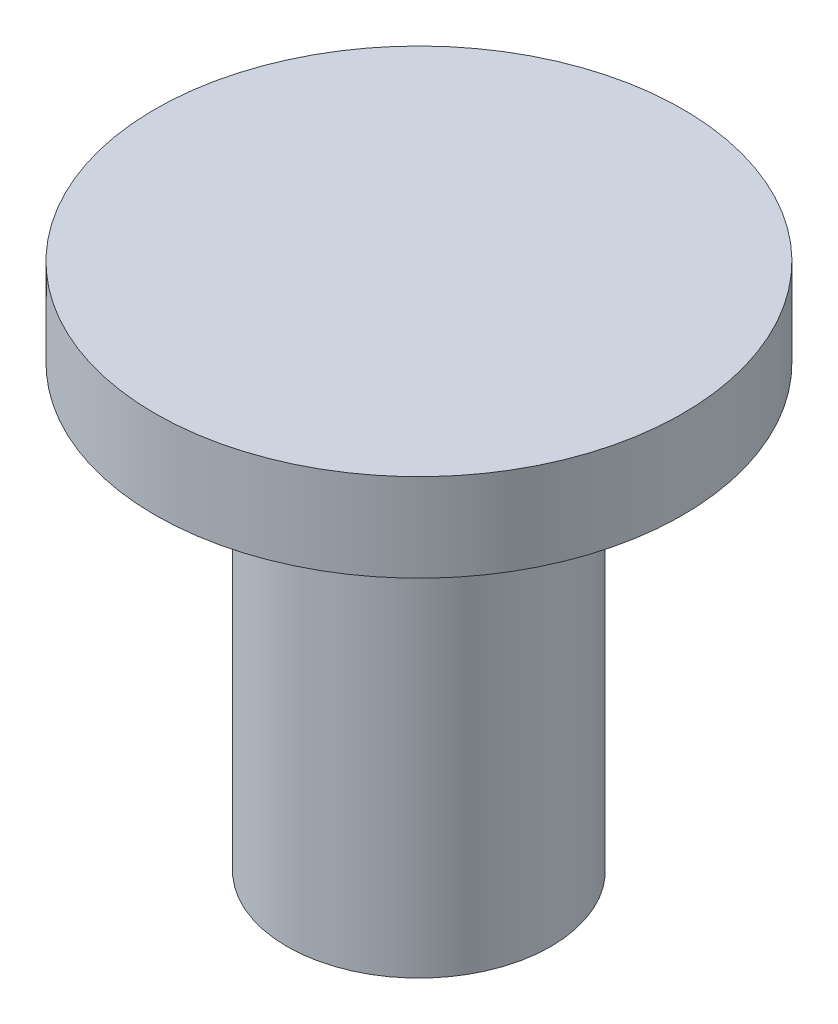
from build123d import *

# Parameters (mm, degrees)
SHANK_PROFILE_6_R = 3
SHANK_6X10_DEPTH  = 10
HEAD_PROFILE_12_R = 6
HEAD_12X2_DEPTH   = 2


with BuildPart() as part:
    # Shank Profile Ø6 → Shank Ø6x10 (new body)
    with BuildSketch(Plane(origin=(0, 0, 0), x_dir=(1, 0, 0), z_dir=(0, 1, 0))):
        with Locations(Location((0, 0, 0), (0, 0, 270))):
            Circle(SHANK_PROFILE_6_R)
    extrude(amount=SHANK_6X10_DEPTH)

    # Head Profile Ø12 → Head Ø12x2 (add)
    with BuildSketch(Plane(origin=(0, 10, 0), x_dir=(1, 0, 0), z_dir=(0, 1, 0))):
        with Locations(Location((0, 0, 0), (0, 0, 270))):
            Circle(HEAD_PROFILE_12_R)
    extrude(amount=HEAD_12X2_DEPTH)


solid = part.part
